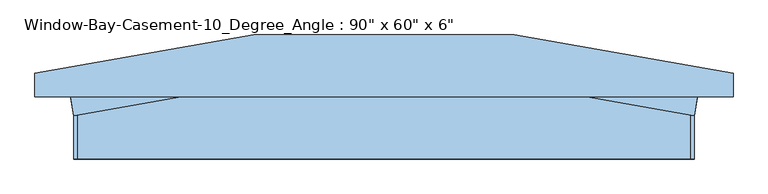
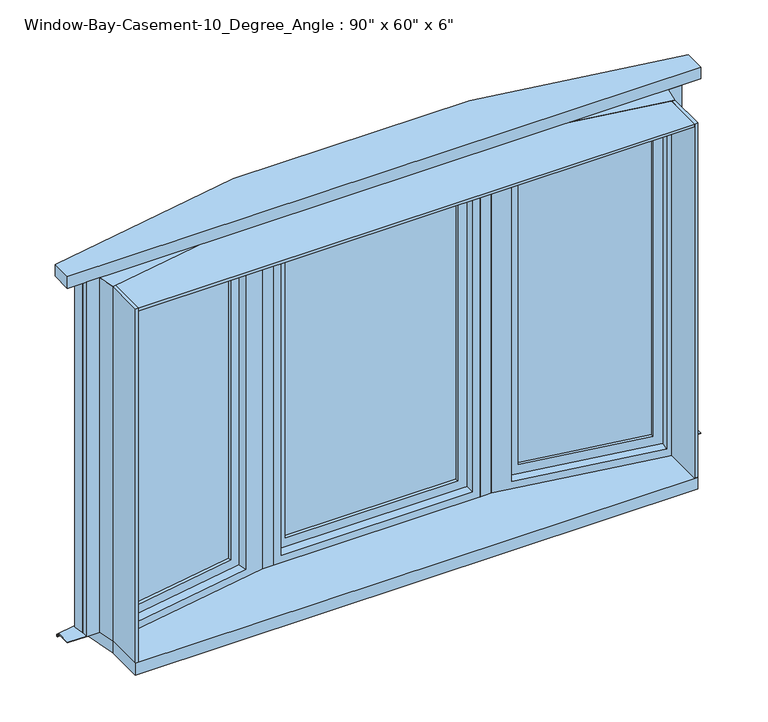
"""IFC4 building model written with IfcOpenShell, lengths in millimetres: window geometry."""

from ifc_helpers import new_model, si_unit, frame, origin, place, context, project, spatial, polyline, outline, extrude, faceted_brep, source, transform, mapped, element, save


def window_bf21e6cb(model_context):
    return source(origin(), model_context, "Body", "SolidModel", [
        extrude(outline(polyline([(1086.3405037, 126.4293252), (1085.2378377, 120.175796), (588.6035631, 207.7458181), (589.7062291, 213.9993474), (1086.3405037, 126.4293252)])), frame((0.0, 0.0, 730.25), z_axis=(0.0, 0.0, 1.0), x_axis=(1.0, 0.0, 0.0)), (0.0, 0.0, 1.0), 1384.3),
        extrude(outline(polyline([(1084.1351718, 113.9222667), (1083.0325059, 107.6687375), (586.3982313, 195.2387597), (587.5008972, 201.4922889), (1084.1351718, 113.9222667)])), frame((0.0, 0.0, 730.25), z_axis=(0.0, 0.0, 1.0), x_axis=(1.0, 0.0, 0.0)), (0.0, 0.0, 1.0), 1384.3),
        extrude(outline(polyline([(1441.45, 57.15), (1441.45, -561.4456588), (-57.15, -561.4456588), (-57.15, 57.15), (1441.45, 57.15)]), holes=[polyline([(1384.3, -504.2956588), (1384.3, 0.0), (0.0, 0.0), (0.0, -504.2956588), (1384.3, -504.2956588)])]), frame((1080.827174, 95.1616791, 730.25), z_axis=(0.17364817766693028, 0.9848077530122081, 0.0), x_axis=(0.0, 0.0, 1.0)), (0.0, 0.0, 1.0), 44.45),
        faceted_brep([(464.7780905, 165.1, 2184.4), (1143.0, 45.5111785, 2184.4), (1155.1293252, 114.3, 2184.4), (1210.6708887, 114.3, 2184.4), (1210.6708887, 136.7463187, 2184.4), (473.6669387, 266.7, 2184.4), (1137.1089371, 85.2376857, 2171.7), (527.9111363, 192.6556946, 2171.7), (538.9377956, 255.1909869, 2171.7), (1148.1355964, 147.772978, 2171.7), (1111.7323538, 51.0245081, 2152.65), (540.0557285, 151.8265214, 2152.65), (546.671724, 189.3476968, 2152.65), (1118.3483494, 88.5456835, 2152.65), (527.9111363, 192.6556946, 673.1), (538.9377956, 255.1909869, 673.1), (540.0557285, 151.8265214, 692.15), (546.671724, 189.3476968, 692.15), (473.6669387, 266.7, 660.4), (1210.6708887, 136.7463187, 660.4), (1210.6708887, 114.3, 660.4), (1155.1293252, 114.3, 660.4), (1143.0, 45.5111785, 660.4), (464.7780905, 165.1, 660.4), (1137.1089371, 85.2376857, 673.1), (1148.1355964, 147.772978, 673.1), (1111.7323538, 51.0245081, 692.15), (1118.3483494, 88.5456835, 692.15)], [[[0, 1, 2, 3, 4, 5]], [[6, 7, 8, 9]], [[10, 11, 12, 13]], [[7, 14, 15, 8]], [[11, 16, 17, 12]], [[18, 19, 20, 21, 22, 23]], [[14, 24, 25, 15]], [[16, 26, 27, 17]], [[22, 21, 2, 1]], [[4, 19, 18, 5], [8, 15, 25, 9]], [[9, 25, 24, 6]], [[6, 24, 14, 7], [12, 17, 27, 13]], [[13, 27, 26, 10]], [[1, 0, 23, 22], [10, 26, 16, 11]], [[5, 18, 23, 0]], [[2, 21, 20, 3]], [[3, 20, 19, 4]]]),
        extrude(outline(polyline([(-1086.3405037, 126.4293252), (-589.7062291, 213.9993474), (-588.6035631, 207.7458181), (-1085.2378377, 120.175796), (-1086.3405037, 126.4293252)])), frame((0.0, 0.0, 730.25), z_axis=(0.0, 0.0, 1.0), x_axis=(1.0, 0.0, 0.0)), (0.0, 0.0, 1.0), 1384.3),
        extrude(outline(polyline([(-1084.1351718, 113.9222667), (-587.5008972, 201.4922889), (-586.3982313, 195.2387597), (-1083.0325059, 107.6687375), (-1084.1351718, 113.9222667)])), frame((0.0, 0.0, 730.25), z_axis=(0.0, 0.0, 1.0), x_axis=(1.0, 0.0, 0.0)), (0.0, 0.0, 1.0), 1384.3),
        extrude(outline(polyline([(1441.45, -57.15), (-57.15, -57.15), (-57.15, 561.4456588), (1441.45, 561.4456588), (1441.45, -57.15)]), holes=[polyline([(1384.3, 504.2956588), (0.0, 504.2956588), (0.0, 0.0), (1384.3, 0.0), (1384.3, 504.2956588)])]), frame((-1080.827174, 95.1616791, 730.25), z_axis=(-0.17364817766693028, 0.9848077530122081, 0.0), x_axis=(0.0, 0.0, 1.0)), (0.0, 0.0, 1.0), 44.45),
        faceted_brep([(-464.7780905, 165.1, 2184.4), (-473.6669387, 266.7, 2184.4), (-1210.6708887, 136.7463187, 2184.4), (-1210.6708887, 114.3, 2184.4), (-1155.1293252, 114.3, 2184.4), (-1143.0, 45.5111785, 2184.4), (-1137.1089371, 85.2376857, 2171.7), (-1148.1355964, 147.772978, 2171.7), (-538.9377956, 255.1909869, 2171.7), (-527.9111363, 192.6556946, 2171.7), (-1111.7323538, 51.0245081, 2152.65), (-1118.3483494, 88.5456835, 2152.65), (-546.671724, 189.3476968, 2152.65), (-540.0557285, 151.8265214, 2152.65), (-538.9377956, 255.1909869, 673.1), (-527.9111363, 192.6556946, 673.1), (-546.671724, 189.3476968, 692.15), (-540.0557285, 151.8265214, 692.15), (-473.6669387, 266.7, 660.4), (-464.7780905, 165.1, 660.4), (-1143.0, 45.5111785, 660.4), (-1155.1293252, 114.3, 660.4), (-1210.6708887, 114.3, 660.4), (-1210.6708887, 136.7463187, 660.4), (-1148.1355964, 147.772978, 673.1), (-1137.1089371, 85.2376857, 673.1), (-1118.3483494, 88.5456835, 692.15), (-1111.7323538, 51.0245081, 692.15)], [[[0, 1, 2, 3, 4, 5]], [[6, 7, 8, 9]], [[10, 11, 12, 13]], [[9, 8, 14, 15]], [[13, 12, 16, 17]], [[18, 19, 20, 21, 22, 23]], [[15, 14, 24, 25]], [[17, 16, 26, 27]], [[20, 5, 4, 21]], [[2, 1, 18, 23], [8, 7, 24, 14]], [[7, 6, 25, 24]], [[6, 9, 15, 25], [12, 11, 26, 16]], [[11, 10, 27, 26]], [[5, 20, 19, 0], [10, 13, 17, 27]], [[1, 0, 19, 18]], [[4, 3, 22, 21]], [[3, 2, 23, 22]]]),
        faceted_brep([(-478.1113628, 317.5, 660.4), (-478.1113628, 317.5, 653.0697935), (478.1113628, 317.5, 653.0697935), (478.1113628, 317.5, 660.4), (-473.6669387, 266.7, 663.1486341), (-473.6669387, 266.7, 660.4), (473.6669387, 266.7, 660.4), (473.6669387, 266.7, 663.1486341), (-478.2335845, 318.897, 654.4483503), (-478.2335845, 318.897, 663.1486341), (478.2335845, 318.897, 663.1486341), (478.2335845, 318.897, 654.4483503), (479.3446905, 331.597, 652.2089977), (-479.3446905, 331.597, 652.2089977), (479.3446905, 331.597, 643.2668038), (-479.3446905, 331.597, 643.2668038), (-478.9980255, 327.6346, 644.7270038), (-478.9980255, 327.6346, 643.2668038), (478.9980255, 327.6346, 643.2668038), (478.9980255, 327.6346, 644.7270038), (-479.2046912, 329.9968, 650.8662705), (-479.2046912, 329.9968, 644.7270038), (479.2046912, 329.9968, 644.7270038), (479.2046912, 329.9968, 650.8662705), (-1286.8726318, 174.8935673, 660.4), (-1286.8726318, 174.8935673, 653.0697935), (1286.8726318, 174.8935673, 660.4), (1286.8726318, 114.3, 660.4), (1210.6726318, 114.3, 660.4), (1210.6726318, 136.7460114, 660.4), (-1210.6726318, 136.7460114, 660.4), (-1210.6726318, 114.3, 660.4), (-1286.8726318, 114.3, 660.4), (-1210.6726318, 136.7460114, 663.1486341), (1210.6726318, 136.7460114, 663.1486341), (1210.6726318, 114.3, 663.1486341), (1286.8726318, 114.3, 663.1486341), (1286.8726318, 176.3121183, 663.1486341), (-1286.8726318, 176.3121183, 663.1486341), (-1286.8726318, 114.3, 663.1486341), (-1210.6726318, 114.3, 663.1486341), (-1286.8726318, 176.3121183, 654.4483503), (-1286.8726318, 189.2080363, 652.2089977), (-1286.8726318, 189.2080363, 643.2668038), (1286.8726318, 189.2080363, 643.2668038), (1286.8726318, 185.1845099, 643.2668038), (-1286.8726318, 185.1845099, 643.2668038), (-1286.8726318, 185.1845099, 644.7270038), (1286.8726318, 185.1845099, 644.7270038), (1286.8726318, 187.5831506, 644.7270038), (-1286.8726318, 187.5831506, 644.7270038), (-1286.8726318, 187.5831506, 650.8662705), (1286.8726318, 174.8935673, 653.0697935), (1286.8726318, 176.3121183, 654.4483503), (1286.8726318, 189.2080363, 652.2089977), (1286.8726318, 187.5831506, 650.8662705)], [[[0, 1, 2, 3]], [[4, 5, 6, 7]], [[8, 9, 10, 11]], [[8, 11, 12, 13]], [[13, 12, 14, 15]], [[16, 17, 18, 19]], [[20, 21, 22, 23]], [[2, 1, 20, 23]], [[1, 0, 24, 25]], [[0, 3, 26, 27, 28, 29, 6, 5, 30, 31, 32, 24]], [[5, 4, 33, 30]], [[4, 7, 34, 35, 36, 37, 10, 9, 38, 39, 40, 33]], [[9, 8, 41, 38]], [[8, 13, 42, 41]], [[13, 15, 43, 42]], [[15, 14, 44, 45, 18, 17, 46, 43]], [[17, 16, 47, 46]], [[16, 19, 48, 49, 22, 21, 50, 47]], [[21, 20, 51, 50]], [[20, 1, 25, 51]], [[3, 2, 52, 26]], [[7, 6, 29, 34]], [[11, 10, 37, 53]], [[12, 11, 53, 54]], [[14, 12, 54, 44]], [[19, 18, 45, 48]], [[23, 22, 49, 55]], [[2, 23, 55, 52]], [[25, 24, 32, 39, 38, 41, 42, 43, 46, 47, 50, 51]], [[27, 26, 52, 55, 49, 48, 45, 44, 54, 53, 37, 36]], [[33, 40, 31, 30]], [[40, 39, 32, 31]], [[36, 35, 28, 27]], [[35, 34, 29, 28]]]),
        extrude(outline(polyline([(-1179.4049856, 142.259341), (-1210.6726318, 136.7460114), (-1218.3912933, 180.520716), (-1187.1236471, 186.0340456), (-1179.4049856, 142.259341)])), frame((0.0, 0.0, 663.1486341), z_axis=(0.0, 0.0, 1.0), x_axis=(1.0, 0.0, 0.0)), (0.0, 0.0, 1.0), 1521.2513659),
        extrude(outline(polyline([(1179.4049856, 142.259341), (1187.1236471, 186.0340456), (1218.3912933, 180.520716), (1210.6726318, 136.7460114), (1179.4049856, 142.259341)])), frame((0.0, 0.0, 663.1486341), z_axis=(0.0, 0.0, 1.0), x_axis=(1.0, 0.0, 0.0)), (0.0, 0.0, 1.0), 1521.2513659),
        extrude(outline(polyline([(480.3335749, 342.9), (1286.8726318, 200.6854033), (1286.8726318, 114.3), (-1286.8708887, 114.3), (-1286.8708887, 200.6857106), (-480.3335749, 342.9), (480.3335749, 342.9)])), frame((0.0, 0.0, 2184.4), z_axis=(0.0, 0.0, 1.0), x_axis=(1.0, 0.0, 0.0)), (0.0, 0.0, 1.0), 50.8),
        extrude(outline(polyline([(-420.0891737, 266.7), (-420.0891737, 165.1), (-464.7780905, 165.1), (-473.6669387, 266.7), (-420.0891737, 266.7)])), frame((0.0, 0.0, 660.4), z_axis=(0.0, 0.0, 1.0), x_axis=(1.0, 0.0, 0.0)), (0.0, 0.0, 1.0), 1524.0),
        extrude(outline(polyline([(473.6669387, 266.7), (464.7780905, 165.1), (420.0891737, 165.1), (420.0891737, 266.7), (473.6669387, 266.7)])), frame((0.0, 0.0, 660.4), z_axis=(0.0, 0.0, 1.0), x_axis=(1.0, 0.0, 0.0)), (0.0, 0.0, 1.0), 1524.0),
        faceted_brep([(407.3891737, 203.2, 673.1), (407.3891737, 266.7, 673.1), (-407.3891737, 266.7, 673.1), (-407.3891737, 203.2, 673.1), (388.3391737, 165.1, 692.15), (388.3391737, 203.2, 692.15), (-388.3391737, 203.2, 692.15), (-388.3391737, 165.1, 692.15), (420.0891737, 266.7, 660.4), (420.0891737, 165.1, 660.4), (-420.0891737, 165.1, 660.4), (-420.0891737, 266.7, 660.4), (-407.3891737, 266.7, 2171.7), (-407.3891737, 203.2, 2171.7), (-388.3391737, 203.2, 2152.65), (-388.3391737, 165.1, 2152.65), (-420.0891737, 165.1, 2184.4), (-420.0891737, 266.7, 2184.4), (407.3891737, 266.7, 2171.7), (407.3891737, 203.2, 2171.7), (388.3391737, 203.2, 2152.65), (388.3391737, 165.1, 2152.65), (420.0891737, 165.1, 2184.4), (420.0891737, 266.7, 2184.4)], [[[0, 1, 2, 3]], [[4, 5, 6, 7]], [[8, 9, 10, 11]], [[3, 2, 12, 13]], [[7, 6, 14, 15]], [[11, 10, 16, 17]], [[13, 12, 18, 19]], [[15, 14, 20, 21]], [[17, 16, 22, 23]], [[11, 17, 23, 8], [1, 18, 12, 2]], [[19, 18, 1, 0]], [[3, 13, 19, 0], [5, 20, 14, 6]], [[21, 20, 5, 4]], [[9, 22, 16, 10], [7, 15, 21, 4]], [[23, 22, 9, 8]]]),
        extrude(outline(polyline([(350.2391737, 234.95), (350.2391737, 228.6), (-350.2391737, 228.6), (-350.2391737, 234.95), (350.2391737, 234.95)])), frame((0.0, 0.0, 730.25), z_axis=(0.0, 0.0, 1.0), x_axis=(1.0, 0.0, 0.0)), (0.0, 0.0, 1.0), 1384.3),
        extrude(outline(polyline([(350.2391737, 222.25), (350.2391737, 215.9), (-350.2391737, 215.9), (-350.2391737, 222.25), (350.2391737, 222.25)])), frame((0.0, 0.0, 730.25), z_axis=(0.0, 0.0, 1.0), x_axis=(1.0, 0.0, 0.0)), (0.0, 0.0, 1.0), 1384.3),
        extrude(outline(polyline([(1143.0, -114.3), (-1143.0, -114.3), (-1143.0, 45.5111785), (-1169.4639823, 195.59588), (-478.1113628, 317.5), (478.1113628, 317.5), (1169.4639823, 195.59588), (1143.0, 45.5111785), (1143.0, -114.3)])), frame((0.0, 0.0, 609.6), z_axis=(0.0, 0.0, 1.0), x_axis=(1.0, 0.0, 0.0)), (0.0, 0.0, 1.0), 50.8),
        extrude(outline(polyline([(2171.7, -407.3891737), (673.1, -407.3891737), (673.1, 407.3891737), (2171.7, 407.3891737), (2171.7, -407.3891737)]), holes=[polyline([(2114.55, 350.2391737), (730.25, 350.2391737), (730.25, -350.2391737), (2114.55, -350.2391737), (2114.55, 350.2391737)])]), frame((0.0, 203.2, 0.0), z_axis=(0.0, 1.0, 0.0), x_axis=(0.0, 0.0, 1.0)), (0.0, 0.0, 1.0), 44.45),
        extrude(outline(polyline([(-1143.0, -114.3), (-1143.0, 45.5111785), (-1130.3, 47.7505311), (-1130.3, -114.3), (-1143.0, -114.3)])), frame((0.0, 0.0, 660.4), z_axis=(0.0, 0.0, 1.0), x_axis=(1.0, 0.0, 0.0)), (0.0, 0.0, 1.0), 1524.0),
        extrude(outline(polyline([(1143.0, -114.3), (1130.3, -114.3), (1130.3, 47.7505311), (1143.0, 45.5111785), (1143.0, -114.3)])), frame((0.0, 0.0, 660.4), z_axis=(0.0, 0.0, 1.0), x_axis=(1.0, 0.0, 0.0)), (0.0, 0.0, 1.0), 1524.0),
        extrude(outline(polyline([(-464.7780905, 165.1), (464.7780905, 165.1), (1130.3, 47.7505311), (1130.3, -114.3), (-1130.3, -114.3), (-1130.3, 47.7505311), (-464.7780905, 165.1)])), frame((0.0, 0.0, 2171.7), z_axis=(0.0, 0.0, 1.0), x_axis=(1.0, 0.0, 0.0)), (0.0, 0.0, 1.0), 12.7),
    ])


if __name__ == "__main__":
    model = new_model("IFC4")
    model_context = context("Model", 3, world=origin())
    ifc_project = project(units=[si_unit("LENGTHUNIT", "METRE", prefix="MILLI")], contexts=[model_context])
    site = spatial("IfcSite", under=ifc_project)
    building = spatial("IfcBuilding", under=site)
    placement = place(None, origin())
    window_shape = window_bf21e6cb(model_context)
    element("IfcWindow", 1, ObjectType="Window-Bay-Casement-10_Degree_Angle : 90\" x 60\" x 6\"", at=placement, inside=building, context=model_context, shape_type="MappedRepresentation", body=[
        mapped(window_shape, transform((0.0, 0.0, 0.0), x_axis=(1.0, 0.0, 0.0), y_axis=(0.0, 1.0, 0.0), z_axis=(0.0, 0.0, 1.0))),
    ])
    save(model, "model.ifc")

# Revit data of these elements
# Type "Window-Bay-Casement-10_Degree_Angle : 90\" x 60\" x 6\""
#   Type Mark = "18"
#   Fire Rating = "0.5h"
#   Assembly Code = "B2020100"
#   Analytic Construction = "Double glazing - domestic"
#   Width of Middle Sash = 2' - 9.07789"
#   Width = 7' - 6"
#   Visual Light Transmittance = 0.81
#   Thermal Resistance (R) = 1.8146 (h·ft²·°F)/BTU
#   Solar Heat Gain Coefficient = 0.76
#   Rough Width = 7' - 6 1/2"
#   Rough Height = 5' - 0 1/2"
#   Length 4 = 0' - 0.24059"
#   Length 3 = 0' - 0 7/64"
#   Length 2 = 3' - 1.29661"
#   Length 1 = 2' - 2.46106"
#   Wall Thickness [instance default] = 0' - 6"
#   Trim Width = 7' - 10.21872"
#   Trim Height = 5' - 0"
#   Height 1 = 5' - 2"
#   Height = 5' - 0"
#   Heat Transfer Coefficient (U) = 0.5511 BTU/(h·ft²·°F)
#   Depth = 0' - 6"
#   Default Sill Height = 2' - 0"
#   Angle 1 = 5.00°
#   Angle = 10.00°
#   Center Muntin Visibility = yes
#   Side Muntin Visibility = yes
#   Interior Trim Visibility [instance default] = yes
#   Exterior Trim Visibility [instance default] = yes
#   Center Muntin Pattern = Muntin Pattern_2x2 : Muntin Pattern_2x2
#   Side Muntin Pattern = Muntin Pattern_2x2 : Muntin Pattern_2x2
#   Interior Trim Material = Wood - Stained
#   Exterior Trim Material = Clad - White
#   Exterior Trim = element 390327
#   Interior Trim = Trim-Window-Interior-Flat : Picture Frame
#   Interior Frame Material = Wood - Stained
#   Glass Panel Material = Glass
#   Exterior Frame Material = Clad - White
#   Wall Closure = (empty or 0)
# Element 1 (IfcWindow, "Window-Bay-Casement-10_Degree_Angle : 90\" x 60\" x 6\"")
#   Wall Thickness = 0' - 9"
#   Materials on its faces: "Clad - White", "Wood - Stained", "Glass"
# Materials
#   "Wood - Stained": class "Wood", colour RGB 224 178 126, transparency 0, Cost = 0
#   "Clad - White": class "Wood", colour RGB 242 242 238, transparency 0, Cost = 0
#   "Glass": class "Glass", colour RGB 0 128 192, transparency 0.75, Description = "Soda Lime Glass", Cost = 0
